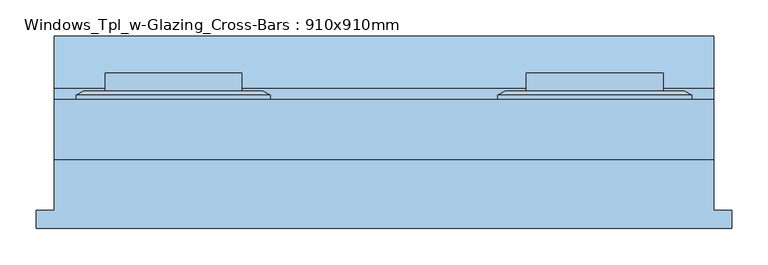
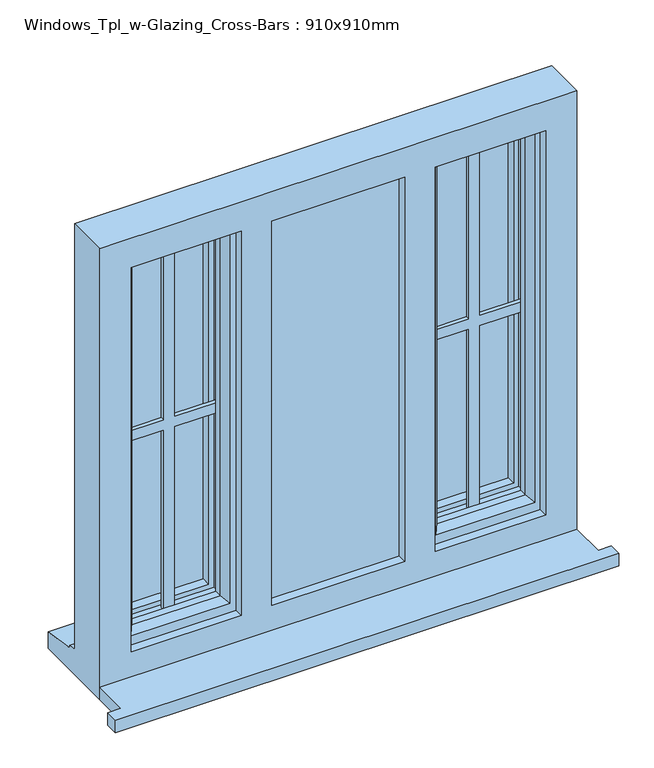
"""IFC4 building model written with IfcOpenShell, lengths in millimetres: window geometry, Windows_Tpl_w-Glazing_Cross-Bars : 910x910mm."""

from ifc_helpers import new_model, si_unit, frame, origin, place, context, project, spatial, polyline, outline, extrude, faceted_brep, source, transform, mapped, element, save


def windows_tpl_w_glazing_cross_bars_910x910mm_4aa0f884(model_context):
    return source(origin(), model_context, "Body", "SolidModel", [
        extrude(outline(polyline([(-906.6666667, -118.1434322), (-906.6666667, -93.1434322), (-881.6666667, -93.1434322), (-881.6666667, -22.9434322), (28.3333333, -22.9434322), (28.3333333, -93.1434322), (53.3333333, -93.1434322), (53.3333333, -118.1434322), (-906.6666667, -118.1434322)])), frame((0.0, 0.0, 1200.0), z_axis=(0.0, 0.0, 1.0), x_axis=(1.0, 0.0, 0.0)), (0.0, 0.0, 1.0), 25.0),
        faceted_brep([(-270.0, 60.0565678, 2080.0), (-270.0, 65.8300705, 2080.0), (-270.0, 65.8300705, 1253.0), (-270.0, 60.0565678, 1253.0), (-260.0, -4.9434322, 2070.0), (-260.0, 60.0565678, 2070.0), (-260.0, 60.0565678, 1263.0), (-260.0, -4.9434322, 1263.0), (-220.0, 9.5494677, 2030.0), (-230.1480377, -4.9434322, 2040.1480377), (-230.1480377, -4.9434322, 1292.8519623), (-220.0, 9.5494677, 1303.0), (-220.0, 24.0565678, 2030.0), (-220.0, 24.0565678, 1303.0), (-230.0, 48.0565678, 2040.0), (-230.0, 24.0565678, 2040.0), (-230.0, 24.0565678, 1293.0), (-230.0, 48.0565678, 1293.0), (-220.0, 65.8300705, 2030.0), (-220.0, 48.0565678, 2030.0), (-220.0, 48.0565678, 1303.0), (-220.0, 65.8300705, 1303.0), (-237.4457548, 71.6035732, 2047.4457548), (-237.4457548, 71.6035732, 1285.5542452), (-259.2153903, 71.6035732, 2069.2153903), (-259.2153903, 71.6035732, 1263.7846097), (-1.6666667, 65.8300705, 1253.0), (-1.6666667, 60.0565678, 1253.0), (-11.6666667, 60.0565678, 1263.0), (-11.6666667, -4.9434322, 1263.0), (-41.5186289, -4.9434322, 1292.8519623), (-51.6666667, 9.5494677, 1303.0), (-51.6666667, 24.0565678, 1303.0), (-41.6666667, 24.0565678, 1293.0), (-41.6666667, 48.0565678, 1293.0), (-51.6666667, 48.0565678, 1303.0), (-51.6666667, 65.8300705, 1303.0), (-34.2209119, 71.6035732, 1285.5542452), (-12.4512764, 71.6035732, 1263.7846097), (-1.6666667, 65.8300705, 2080.0), (-1.6666667, 60.0565678, 2080.0), (-11.6666667, 60.0565678, 2070.0), (-11.6666667, -4.9434322, 2070.0), (-41.5186289, -4.9434322, 2040.1480377), (-51.6666667, 9.5494677, 2030.0), (-51.6666667, 24.0565678, 2030.0), (-41.6666667, 24.0565678, 2040.0), (-41.6666667, 48.0565678, 2040.0), (-51.6666667, 48.0565678, 2030.0), (-51.6666667, 65.8300705, 2030.0), (-34.2209119, 71.6035732, 2047.4457548), (-12.4512764, 71.6035732, 2069.2153903)], [[[0, 1, 2, 3]], [[4, 5, 6, 7]], [[8, 9, 10, 11]], [[12, 8, 11, 13]], [[14, 15, 16, 17]], [[18, 19, 20, 21]], [[22, 18, 21, 23]], [[1, 24, 25, 2]], [[3, 2, 26, 27]], [[7, 6, 28, 29]], [[11, 10, 30, 31]], [[13, 11, 31, 32]], [[17, 16, 33, 34]], [[21, 20, 35, 36]], [[23, 21, 36, 37]], [[2, 25, 38, 26]], [[27, 26, 39, 40]], [[29, 28, 41, 42]], [[31, 30, 43, 44]], [[32, 31, 44, 45]], [[34, 33, 46, 47]], [[36, 35, 48, 49]], [[37, 36, 49, 50]], [[26, 38, 51, 39]], [[40, 39, 1, 0]], [[3, 27, 40, 0], [5, 41, 28, 6]], [[42, 41, 5, 4]], [[7, 29, 42, 4], [9, 43, 30, 10]], [[44, 43, 9, 8]], [[45, 44, 8, 12]], [[15, 46, 33, 16], [13, 32, 45, 12]], [[47, 46, 15, 14]], [[17, 34, 47, 14], [19, 48, 35, 20]], [[49, 48, 19, 18]], [[50, 49, 18, 22]], [[24, 51, 38, 25], [23, 37, 50, 22]], [[39, 51, 24, 1]]]),
        faceted_brep([(-583.3333333, 60.0565678, 2080.0), (-583.3333333, 65.8300705, 2080.0), (-851.6666667, 65.8300705, 2080.0), (-851.6666667, 60.0565678, 2080.0), (-593.3333333, -4.9434322, 2070.0), (-593.3333333, 60.0565678, 2070.0), (-841.6666667, 60.0565678, 2070.0), (-841.6666667, -4.9434322, 2070.0), (-633.3333333, 9.5494677, 2030.0), (-623.1852956, -4.9434322, 2040.1480377), (-811.8147044, -4.9434322, 2040.1480377), (-801.6666667, 9.5494677, 2030.0), (-633.3333333, 24.0565678, 2030.0), (-801.6666667, 24.0565678, 2030.0), (-623.3333333, 48.0565678, 2040.0), (-623.3333333, 24.0565678, 2040.0), (-811.6666667, 24.0565678, 2040.0), (-811.6666667, 48.0565678, 2040.0), (-633.3333333, 65.8300705, 2030.0), (-633.3333333, 48.0565678, 2030.0), (-801.6666667, 48.0565678, 2030.0), (-801.6666667, 65.8300705, 2030.0), (-615.8875785, 71.6035732, 2047.4457548), (-819.1124215, 71.6035732, 2047.4457548), (-594.117943, 71.6035732, 2069.2153903), (-840.882057, 71.6035732, 2069.2153903), (-851.6666667, 65.8300705, 1253.0), (-851.6666667, 60.0565678, 1253.0), (-841.6666667, 60.0565678, 1263.0), (-841.6666667, -4.9434322, 1263.0), (-811.8147044, -4.9434322, 1292.8519623), (-801.6666667, 9.5494677, 1303.0), (-801.6666667, 24.0565678, 1303.0), (-811.6666667, 24.0565678, 1293.0), (-811.6666667, 48.0565678, 1293.0), (-801.6666667, 48.0565678, 1303.0), (-801.6666667, 65.8300705, 1303.0), (-819.1124215, 71.6035732, 1285.5542452), (-840.882057, 71.6035732, 1263.7846097), (-583.3333333, 65.8300705, 1253.0), (-583.3333333, 60.0565678, 1253.0), (-593.3333333, 60.0565678, 1263.0), (-593.3333333, -4.9434322, 1263.0), (-623.1852956, -4.9434322, 1292.8519623), (-633.3333333, 9.5494677, 1303.0), (-633.3333333, 24.0565678, 1303.0), (-623.3333333, 24.0565678, 1293.0), (-623.3333333, 48.0565678, 1293.0), (-633.3333333, 48.0565678, 1303.0), (-633.3333333, 65.8300705, 1303.0), (-615.8875785, 71.6035732, 1285.5542452), (-594.117943, 71.6035732, 1263.7846097)], [[[0, 1, 2, 3]], [[4, 5, 6, 7]], [[8, 9, 10, 11]], [[12, 8, 11, 13]], [[14, 15, 16, 17]], [[18, 19, 20, 21]], [[22, 18, 21, 23]], [[1, 24, 25, 2]], [[3, 2, 26, 27]], [[7, 6, 28, 29]], [[11, 10, 30, 31]], [[13, 11, 31, 32]], [[17, 16, 33, 34]], [[21, 20, 35, 36]], [[23, 21, 36, 37]], [[2, 25, 38, 26]], [[27, 26, 39, 40]], [[0, 3, 27, 40], [41, 28, 6, 5]], [[29, 28, 41, 42]], [[4, 7, 29, 42], [43, 30, 10, 9]], [[31, 30, 43, 44]], [[32, 31, 44, 45]], [[46, 33, 16, 15], [12, 13, 32, 45]], [[34, 33, 46, 47]], [[14, 17, 34, 47], [48, 35, 20, 19]], [[36, 35, 48, 49]], [[37, 36, 49, 50]], [[51, 38, 25, 24], [22, 23, 37, 50]], [[26, 38, 51, 39]], [[40, 39, 1, 0]], [[42, 41, 5, 4]], [[44, 43, 9, 8]], [[45, 44, 8, 12]], [[47, 46, 15, 14]], [[49, 48, 19, 18]], [[50, 49, 18, 22]], [[39, 51, 24, 1]]]),
        extrude(outline(polyline([(1293.0, -145.8333333), (1293.0, -125.8333333), (1656.5, -125.8333333), (1656.5, -41.6666667), (1676.5, -41.6666667), (1676.5, -125.8333333), (2040.1480377, -125.8333333), (2040.1480377, -145.8333333), (1676.5, -145.8333333), (1676.5, -230.1480377), (1656.5, -230.1480377), (1656.5, -145.8333333), (1293.0, -145.8333333)])), frame((0.0, 32.0565678, 0.0), z_axis=(0.0, 1.0, 0.0), x_axis=(0.0, 0.0, 1.0)), (0.0, 0.0, 1.0), 8.0),
        extrude(outline(polyline([(1293.0, -727.5), (1293.0, -707.5), (1656.5, -707.5), (1656.5, -623.3333333), (1676.5, -623.3333333), (1676.5, -707.5), (2040.1480377, -707.5), (2040.1480377, -727.5), (1676.5, -727.5), (1676.5, -811.6666667), (1656.5, -811.6666667), (1656.5, -727.5), (1293.0, -727.5)])), frame((0.0, 32.0565678, 0.0), z_axis=(0.0, 1.0, 0.0), x_axis=(0.0, 0.0, 1.0)), (0.0, 0.0, 1.0), 8.0),
        extrude(outline(polyline([(1263.0, -436.6666667), (1263.0, -416.6666667), (1656.5, -416.6666667), (1656.5, -290.0), (1676.5, -290.0), (1676.5, -416.6666667), (2070.0, -416.6666667), (2070.0, -436.6666667), (1676.5, -436.6666667), (1676.5, -563.3333333), (1656.5, -563.3333333), (1656.5, -436.6666667), (1263.0, -436.6666667)])), frame((0.0, 3.0565678, 0.0), z_axis=(0.0, 1.0, 0.0), x_axis=(0.0, 0.0, 1.0)), (0.0, 0.0, 1.0), 8.0),
        faceted_brep([(28.3333333, -22.9434322, 2110.0), (-881.6666667, -22.9434322, 2110.0), (-881.6666667, -22.9434322, 1200.0), (28.3333333, -22.9434322, 1200.0), (-31.6666667, -22.9434322, 2050.0), (-31.6666667, -22.9434322, 1275.0), (-242.0, -22.9434322, 1275.0), (-242.0, -22.9434322, 2050.0), (-300.0, -22.9434322, 2050.0), (-300.0, -22.9434322, 1275.0), (-553.3333333, -22.9434322, 1275.0), (-553.3333333, -22.9434322, 2050.0), (-611.3333333, -22.9434322, 2050.0), (-611.3333333, -22.9434322, 1275.0), (-821.6666667, -22.9434322, 1275.0), (-821.6666667, -22.9434322, 2050.0), (-881.6666667, 60.0565678, 2110.0), (-881.6666667, 60.0565678, 1251.0), (-881.6666667, 75.0565678, 1249.68767), (-881.6666667, 75.0565678, 1244.7449676), (-881.6666667, 147.5565678, 1233.8088847), (-881.6666667, 147.5565678, 1200.0), (28.3333333, 60.0565678, 2110.0), (28.3333333, 60.0565678, 1251.0), (-841.6666667, 60.0565678, 2070.0), (-841.6666667, 60.0565678, 1263.0), (-593.3333333, 60.0565678, 1263.0), (-593.3333333, 60.0565678, 2070.0), (-553.3333333, 60.0565678, 2070.0), (-553.3333333, 60.0565678, 1263.0), (-300.0, 60.0565678, 1263.0), (-300.0, 60.0565678, 2070.0), (-260.0, 60.0565678, 2070.0), (-260.0, 60.0565678, 1263.0), (-11.6666667, 60.0565678, 1263.0), (-11.6666667, 60.0565678, 2070.0), (-841.6666667, -4.9434322, 2070.0), (-841.6666667, -4.9434322, 1263.0), (-563.3333333, -4.9434322, 2070.0), (-290.0, -4.9434322, 2070.0), (-290.0, -4.9434322, 1263.0), (-563.3333333, -4.9434322, 1263.0), (-300.0, -4.9434322, 2050.0), (-553.3333333, -4.9434322, 2050.0), (-553.3333333, -4.9434322, 1275.0), (-300.0, -4.9434322, 1275.0), (-260.0, -4.9434322, 2070.0), (-11.6666667, -4.9434322, 2070.0), (-11.6666667, -4.9434322, 1263.0), (-260.0, -4.9434322, 1263.0), (-31.6666667, -4.9434322, 2050.0), (-242.0, -4.9434322, 2050.0), (-242.0, -4.9434322, 1275.0), (-31.6666667, -4.9434322, 1275.0), (-593.3333333, -4.9434322, 2070.0), (-593.3333333, -4.9434322, 1263.0), (-611.3333333, -4.9434322, 2050.0), (-821.6666667, -4.9434322, 2050.0), (-821.6666667, -4.9434322, 1275.0), (-611.3333333, -4.9434322, 1275.0), (-553.3333333, 19.0565678, 2070.0), (-300.0, 19.0565678, 2070.0), (-290.0, 19.0565678, 2070.0), (-563.3333333, 19.0565678, 2070.0), (28.3333333, 147.5565678, 1200.0), (28.3333333, 147.5565678, 1233.8088847), (28.3333333, 75.0565678, 1244.7449676), (28.3333333, 75.0565678, 1249.68767), (-553.3333333, 19.0565678, 1263.0), (-563.3333333, 19.0565678, 1263.0), (-290.0, 19.0565678, 1263.0), (-300.0, 19.0565678, 1263.0)], [[[0, 1, 2, 3], [4, 5, 6, 7], [8, 9, 10, 11], [12, 13, 14, 15]], [[2, 1, 16, 17, 18, 19, 20, 21]], [[17, 16, 22, 23], [24, 25, 26, 27], [28, 29, 30, 31], [32, 33, 34, 35]], [[25, 24, 36, 37]], [[38, 39, 40, 41], [42, 43, 44, 45]], [[46, 47, 48, 49], [50, 51, 52, 53]], [[36, 54, 55, 37], [56, 57, 58, 59]], [[57, 15, 14, 58]], [[1, 0, 22, 16]], [[36, 24, 27, 54]], [[35, 47, 46, 32]], [[60, 28, 31, 61, 62, 39, 38, 63]], [[15, 57, 56, 12]], [[50, 4, 7, 51]], [[11, 43, 42, 8]], [[23, 22, 0, 3, 64, 65, 66, 67]], [[35, 34, 48, 47]], [[4, 50, 53, 5]], [[43, 11, 10, 44]], [[12, 56, 59, 13]], [[27, 26, 55, 54]], [[29, 28, 60, 68]], [[68, 60, 63, 69]], [[69, 63, 38, 41]], [[62, 70, 40, 39]], [[70, 62, 61, 71]], [[71, 61, 31, 30]], [[33, 32, 46, 49]], [[51, 7, 6, 52]], [[8, 42, 45, 9]], [[64, 3, 2, 21]], [[65, 64, 21, 20]], [[66, 65, 20, 19]], [[67, 66, 19, 18]], [[23, 67, 18, 17]], [[26, 25, 37, 55]], [[34, 33, 49, 48]], [[41, 40, 70, 71, 30, 29, 68, 69]], [[6, 5, 53, 52]], [[45, 44, 10, 9]], [[59, 58, 14, 13]]]),
        extrude(outline(polyline([(-563.3333333, 19.0565678), (-290.0, 19.0565678), (-290.0, -4.9434322), (-563.3333333, -4.9434322), (-563.3333333, 19.0565678)])), frame((0.0, 0.0, 1263.0), z_axis=(0.0, 0.0, 1.0), x_axis=(1.0, 0.0, 0.0)), (0.0, 0.0, 1.0), 807.0),
        extrude(outline(polyline([(-623.3333333, 72.4565678), (-811.6666667, 72.4565678), (-811.6666667, 96.4565678), (-623.3333333, 96.4565678), (-623.3333333, 72.4565678)])), frame((0.0, 0.0, 1293.0), z_axis=(0.0, 0.0, 1.0), x_axis=(1.0, 0.0, 0.0)), (0.0, 0.0, 1.0), 747.0),
        extrude(outline(polyline([(-41.5186289, 72.4565678), (-230.1480377, 72.4565678), (-230.1480377, 96.4565678), (-41.5186289, 96.4565678), (-41.5186289, 72.4565678)])), frame((0.0, 0.0, 1292.8519623), z_axis=(0.0, 0.0, 1.0), x_axis=(1.0, 0.0, 0.0)), (0.0, 0.0, 1.0), 747.2960754),
    ])


if __name__ == "__main__":
    model = new_model("IFC4")
    model_context = context("Model", 3, world=origin())
    ifc_project = project(units=[si_unit("LENGTHUNIT", "METRE", prefix="MILLI")], contexts=[model_context])
    site = spatial("IfcSite", under=ifc_project)
    building = spatial("IfcBuilding", under=site)
    placement = place(None, origin())
    windows_tpl_w_glazing_cross_bars_910x910mm_shape = windows_tpl_w_glazing_cross_bars_910x910mm_4aa0f884(model_context)
    element("IfcWindow", 1, ObjectType="Windows_Tpl_w-Glazing_Cross-Bars : 910x910mm", at=placement, inside=building, context=model_context, shape_type="MappedRepresentation", body=[
        mapped(windows_tpl_w_glazing_cross_bars_910x910mm_shape, transform((0.0, 0.0, 0.0), x_axis=(1.0, 0.0, 0.0), y_axis=(0.0, 1.0, 0.0), z_axis=(0.0, 0.0, 1.0))),
    ])
    save(model, "model.ifc")

# Revit data of these elements
# Type "Windows_Tpl_w-Glazing_Cross-Bars : 910x910mm"
#   Type Mark = "18"
#   Operation = "TriplePanelVertical"
#   Construction Type Id = "GSP4R"
#   Manufacturer = "Revit"
#   Keynote = "L10"
#   Analytic Construction = "1/8 in Pilkington single glazing"
#   Wrap Layers (Ext) from Ext = 0' - 4.03543"
#   Wrap Layers (Int) from Ext = 0' - 6.98819"
#   Window Board Projection = 0' - 0.98425"
#   Window Board Extension = 0' - 0.98425"
#   Visual Light Transmittance = 0.9
#   Solar Heat Gain Coefficient = 0.78
#   Rough Width = 2' - 11.82677"
#   Rough Height = 2' - 11.82677"
#   Height = 2' - 11.82677"
#   Width = 2' - 11.82677"
#   Heat Transfer Coefficient (U) = 0.6496 BTU/(h·ft²·°F)
#   Glazing Thickness = 0' - 0.94488"
#   Glazing Bar Thickness = 0' - 0.7874"
#   FrameOffset - External = 0' - 1.9685"
#   Frame Depth = 0' - 2.55906"
#   Default Head Height = 6' - 11.07087"
#   Cill Depth = 0' - 3.44488"
#   Cavity Closer Width = 0' - 1.9685"
#   Cavity Closer Offset from Ext = 0' - 4.03543"
#   Cavity Closer Depth = 0' - 3.34646"
#   Vis - Glazing Bars = yes
#   Vis - Cavity Closers = yes
#   Define Thermal Properties by = 1
#   Material Trim = Window Frame
#   Material Glazing Bars = Window Frame
#   Material Glass = Glass
#   Material Frame = Window Frame
#   Wall Closure = (empty or 0)
# Element 1 (IfcWindow, "Windows_Tpl_w-Glazing_Cross-Bars : 910x910mm")
#   Materials on its faces: "Window Frame", "Glass"
# Materials
#   "Window Frame": colour RGB 249 249 249, transparency 0
#   "Glass": class "Glass", colour RGB 0 128 192, transparency 0.75, Description = "Soda Lime Glass", Cost = 0
